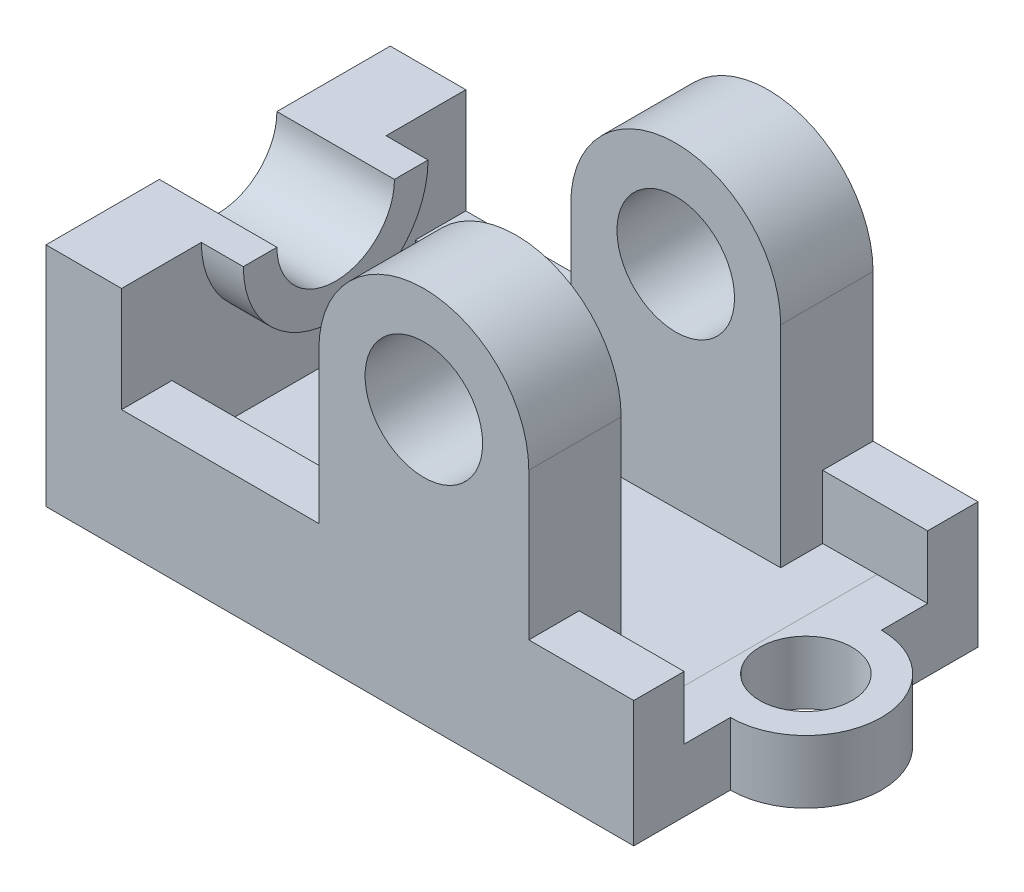
ISO-10303-21;
HEADER;
FILE_DESCRIPTION(('STEP AP214'),'2;1');
FILE_NAME('part.step','',(''),(''),'','','');
FILE_SCHEMA(('AUTOMOTIVE_DESIGN { 1 0 10303 214 1 1 1 1 }'));
ENDSEC;
DATA;
#1=APPLICATION_CONTEXT('core data for automotive mechanical design processes');
#2=APPLICATION_PROTOCOL_DEFINITION('international standard','automotive_design',2000,#1);
#3=PRODUCT_CONTEXT('',#1,'mechanical');
#4=PRODUCT('Part','Part','',(#3));
#5=PRODUCT_RELATED_PRODUCT_CATEGORY('part','',(#4));
#6=PRODUCT_DEFINITION_FORMATION('','',#4);
#7=PRODUCT_DEFINITION_CONTEXT('part definition',#1,'design');
#8=PRODUCT_DEFINITION('design','',#6,#7);
#9=PRODUCT_DEFINITION_SHAPE('','',#8);
#10=(LENGTH_UNIT() NAMED_UNIT(*) SI_UNIT(.MILLI.,.METRE.));
#11=(NAMED_UNIT(*) PLANE_ANGLE_UNIT() SI_UNIT($,.RADIAN.));
#12=(NAMED_UNIT(*) SI_UNIT($,.STERADIAN.) SOLID_ANGLE_UNIT());
#13=UNCERTAINTY_MEASURE_WITH_UNIT(LENGTH_MEASURE(1.E-05),#10,'distance_accuracy_value','');
#14=(GEOMETRIC_REPRESENTATION_CONTEXT(3) GLOBAL_UNCERTAINTY_ASSIGNED_CONTEXT((#13)) GLOBAL_UNIT_ASSIGNED_CONTEXT((#10,
#11,#12)) REPRESENTATION_CONTEXT('',''));
#15=CARTESIAN_POINT('',(0.,0.,0.));
#16=DIRECTION('',(0.,0.,1.));
#17=DIRECTION('',(1.,0.,0.));
#18=AXIS2_PLACEMENT_3D('',#15,#16,#17);
#19=CARTESIAN_POINT('',(0.,54.,82.));
#20=DIRECTION('',(0.,1.,0.));
#21=DIRECTION('',(0.,0.,1.));
#22=AXIS2_PLACEMENT_3D('',#19,#20,#21);
#23=PLANE('',#22);
#24=DIRECTION('',(-1.,0.,0.));
#25=VECTOR('',#24,1.);
#26=CARTESIAN_POINT('',(28.,54.,27.));
#27=LINE('',#26,#25);
#28=CARTESIAN_POINT('',(28.,54.,27.));
#29=VERTEX_POINT('',#28);
#30=CARTESIAN_POINT('',(0.,54.,27.));
#31=VERTEX_POINT('',#30);
#32=EDGE_CURVE('E237',#29,#31,#27,.T.);
#33=ORIENTED_EDGE('',*,*,#32,.F.);
#34=DIRECTION('',(0.,0.,1.));
#35=VECTOR('',#34,1.);
#36=CARTESIAN_POINT('',(28.,54.,63.));
#37=LINE('',#36,#35);
#38=CARTESIAN_POINT('',(28.,54.,19.));
#39=VERTEX_POINT('',#38);
#40=EDGE_CURVE('E247',#39,#29,#37,.T.);
#41=ORIENTED_EDGE('',*,*,#40,.F.);
#42=DIRECTION('',(-1.,0.,0.));
#43=VECTOR('',#42,1.);
#44=CARTESIAN_POINT('',(28.,54.,19.));
#45=LINE('',#44,#43);
#46=CARTESIAN_POINT('',(18.,54.,19.));
#47=VERTEX_POINT('',#46);
#48=EDGE_CURVE('E258',#39,#47,#45,.T.);
#49=ORIENTED_EDGE('',*,*,#48,.T.);
#50=DIRECTION('',(0.,0.,-1.));
#51=VECTOR('',#50,1.);
#52=CARTESIAN_POINT('',(18.,54.,82.));
#53=LINE('',#52,#51);
#54=CARTESIAN_POINT('',(18.,54.,0.));
#55=VERTEX_POINT('',#54);
#56=EDGE_CURVE('E478',#47,#55,#53,.T.);
#57=ORIENTED_EDGE('',*,*,#56,.T.);
#58=DIRECTION('',(1.,0.,0.));
#59=VECTOR('',#58,1.);
#60=CARTESIAN_POINT('',(0.,54.,0.));
#61=LINE('',#60,#59);
#62=CARTESIAN_POINT('',(0.,54.,0.));
#63=VERTEX_POINT('',#62);
#64=EDGE_CURVE('E464',#63,#55,#61,.T.);
#65=ORIENTED_EDGE('',*,*,#64,.F.);
#66=DIRECTION('',(0.,0.,-1.));
#67=VECTOR('',#66,1.);
#68=CARTESIAN_POINT('',(0.,54.,82.));
#69=LINE('',#68,#67);
#70=EDGE_CURVE('E252',#31,#63,#69,.T.);
#71=ORIENTED_EDGE('',*,*,#70,.F.);
#72=EDGE_LOOP('',(#33,#41,#49,#57,#65,#71));
#73=FACE_BOUND('',#72,.T.);
#74=ADVANCED_FACE('F50',(#73),#23,.T.);
#75=CARTESIAN_POINT('',(18.,0.,82.));
#76=DIRECTION('',(1.,0.,0.));
#77=DIRECTION('',(0.,1.,0.));
#78=AXIS2_PLACEMENT_3D('',#75,#76,#77);
#79=PLANE('',#78);
#80=ORIENTED_EDGE('',*,*,#56,.F.);
#81=CARTESIAN_POINT('',(18.,54.,41.));
#82=DIRECTION('',(1.,0.,0.));
#83=DIRECTION('',(0.,1.,0.));
#84=AXIS2_PLACEMENT_3D('',#81,#82,#83);
#85=CIRCLE('',#84,22.);
#86=CARTESIAN_POINT('',(18.,54.,63.));
#87=VERTEX_POINT('',#86);
#88=EDGE_CURVE('E71',#87,#47,#85,.T.);
#89=ORIENTED_EDGE('',*,*,#88,.F.);
#90=CARTESIAN_POINT('',(18.,54.,82.));
#91=VERTEX_POINT('',#90);
#92=EDGE_CURVE('E57',#91,#87,#53,.T.);
#93=ORIENTED_EDGE('',*,*,#92,.F.);
#94=DIRECTION('',(0.,-1.,0.));
#95=VECTOR('',#94,1.);
#96=CARTESIAN_POINT('',(18.,0.,82.));
#97=LINE('',#96,#95);
#98=CARTESIAN_POINT('',(18.,29.,82.));
#99=VERTEX_POINT('',#98);
#100=EDGE_CURVE('E446',#91,#99,#97,.T.);
#101=ORIENTED_EDGE('',*,*,#100,.T.);
#102=DIRECTION('',(0.,0.,1.));
#103=VECTOR('',#102,1.);
#104=CARTESIAN_POINT('',(18.,29.,70.));
#105=LINE('',#104,#103);
#106=CARTESIAN_POINT('',(18.,29.,70.));
#107=VERTEX_POINT('',#106);
#108=EDGE_CURVE('E308',#107,#99,#105,.T.);
#109=ORIENTED_EDGE('',*,*,#108,.F.);
#110=DIRECTION('',(0.,-1.,0.));
#111=VECTOR('',#110,1.);
#112=CARTESIAN_POINT('',(18.,14.,70.));
#113=LINE('',#112,#111);
#114=CARTESIAN_POINT('',(18.,14.,70.));
#115=VERTEX_POINT('',#114);
#116=EDGE_CURVE('E305',#107,#115,#113,.T.);
#117=ORIENTED_EDGE('',*,*,#116,.T.);
#118=DIRECTION('',(0.,0.,-1.));
#119=VECTOR('',#118,1.);
#120=CARTESIAN_POINT('',(18.,14.,82.));
#121=LINE('',#120,#119);
#122=CARTESIAN_POINT('',(18.,14.,12.));
#123=VERTEX_POINT('',#122);
#124=EDGE_CURVE('E11',#115,#123,#121,.T.);
#125=ORIENTED_EDGE('',*,*,#124,.T.);
#126=DIRECTION('',(0.,1.,0.));
#127=VECTOR('',#126,1.);
#128=CARTESIAN_POINT('',(18.,14.,12.));
#129=LINE('',#128,#127);
#130=CARTESIAN_POINT('',(18.,29.,12.));
#131=VERTEX_POINT('',#130);
#132=EDGE_CURVE('E363',#123,#131,#129,.T.);
#133=ORIENTED_EDGE('',*,*,#132,.T.);
#134=DIRECTION('',(0.,0.,-1.));
#135=VECTOR('',#134,1.);
#136=CARTESIAN_POINT('',(18.,29.,12.));
#137=LINE('',#136,#135);
#138=CARTESIAN_POINT('',(18.,29.,0.));
#139=VERTEX_POINT('',#138);
#140=EDGE_CURVE('E367',#131,#139,#137,.T.);
#141=ORIENTED_EDGE('',*,*,#140,.T.);
#142=DIRECTION('',(0.,-1.,0.));
#143=VECTOR('',#142,1.);
#144=CARTESIAN_POINT('',(18.,0.,0.));
#145=LINE('',#144,#143);
#146=EDGE_CURVE('E443',#55,#139,#145,.T.);
#147=ORIENTED_EDGE('',*,*,#146,.F.);
#148=EDGE_LOOP('',(#80,#89,#93,#101,#109,#117,#125,#133,#141,#147));
#149=FACE_BOUND('',#148,.T.);
#150=ADVANCED_FACE('F484',(#149),#79,.T.);
#151=CARTESIAN_POINT('',(140.,0.,0.));
#152=DIRECTION('',(1.,0.,0.));
#153=DIRECTION('',(0.,0.,-1.));
#154=AXIS2_PLACEMENT_3D('',#151,#152,#153);
#155=PLANE('',#154);
#156=DIRECTION('',(0.,1.,0.));
#157=VECTOR('',#156,1.);
#158=CARTESIAN_POINT('',(140.,0.,23.));
#159=LINE('',#158,#157);
#160=CARTESIAN_POINT('',(140.,0.,23.));
#161=VERTEX_POINT('',#160);
#162=CARTESIAN_POINT('',(140.,15.,23.));
#163=VERTEX_POINT('',#162);
#164=EDGE_CURVE('E276',#161,#163,#159,.T.);
#165=ORIENTED_EDGE('',*,*,#164,.F.);
#166=DIRECTION('',(0.,0.,1.));
#167=VECTOR('',#166,1.);
#168=CARTESIAN_POINT('',(140.,0.,0.));
#169=LINE('',#168,#167);
#170=CARTESIAN_POINT('',(140.,0.,0.));
#171=VERTEX_POINT('',#170);
#172=EDGE_CURVE('E447',#171,#161,#169,.T.);
#173=ORIENTED_EDGE('',*,*,#172,.F.);
#174=DIRECTION('',(0.,1.,0.));
#175=VECTOR('',#174,1.);
#176=CARTESIAN_POINT('',(140.,0.,0.));
#177=LINE('',#176,#175);
#178=CARTESIAN_POINT('',(140.,30.,0.));
#179=VERTEX_POINT('',#178);
#180=EDGE_CURVE('E438',#171,#179,#177,.T.);
#181=ORIENTED_EDGE('',*,*,#180,.T.);
#182=DIRECTION('',(0.,0.,-1.));
#183=VECTOR('',#182,1.);
#184=CARTESIAN_POINT('',(140.,30.,12.));
#185=LINE('',#184,#183);
#186=CARTESIAN_POINT('',(140.,30.,12.));
#187=VERTEX_POINT('',#186);
#188=EDGE_CURVE('E350',#187,#179,#185,.T.);
#189=ORIENTED_EDGE('',*,*,#188,.F.);
#190=DIRECTION('',(0.,-1.,0.));
#191=VECTOR('',#190,1.);
#192=CARTESIAN_POINT('',(140.,15.,12.));
#193=LINE('',#192,#191);
#194=CARTESIAN_POINT('',(140.,15.,12.));
#195=VERTEX_POINT('',#194);
#196=EDGE_CURVE('E341',#187,#195,#193,.T.);
#197=ORIENTED_EDGE('',*,*,#196,.T.);
#198=DIRECTION('',(0.,0.,1.));
#199=VECTOR('',#198,1.);
#200=CARTESIAN_POINT('',(140.,15.,0.));
#201=LINE('',#200,#199);
#202=EDGE_CURVE('E445',#195,#163,#201,.T.);
#203=ORIENTED_EDGE('',*,*,#202,.T.);
#204=EDGE_LOOP('',(#165,#173,#181,#189,#197,#203));
#205=FACE_BOUND('',#204,.T.);
#206=ADVANCED_FACE('F513',(#205),#155,.T.);
#207=CARTESIAN_POINT('',(-0.12577472936121,13.8352202297331,82.));
#208=DIRECTION('',(-0.00909053345679159,0.999958680247074,0.));
#209=DIRECTION('',(-0.999958680247075,-0.00909053345679159,0.));
#210=AXIS2_PLACEMENT_3D('',#207,#208,#209);
#211=PLANE('',#210);
#212=DIRECTION('',(0.999958680247074,0.0090905334567916,0.));
#213=VECTOR('',#212,1.);
#214=CARTESIAN_POINT('',(65.,14.4272727272727,70.));
#215=LINE('',#214,#213);
#216=CARTESIAN_POINT('',(65.,14.4272727272727,70.));
#217=VERTEX_POINT('',#216);
#218=EDGE_CURVE('E295',#115,#217,#215,.T.);
#219=ORIENTED_EDGE('',*,*,#218,.T.);
#220=DIRECTION('',(0.,0.,1.));
#221=VECTOR('',#220,1.);
#222=CARTESIAN_POINT('',(65.,14.4272727272727,60.));
#223=LINE('',#222,#221);
#224=CARTESIAN_POINT('',(65.,14.4272727272727,60.));
#225=VERTEX_POINT('',#224);
#226=EDGE_CURVE('E435',#225,#217,#223,.T.);
#227=ORIENTED_EDGE('',*,*,#226,.F.);
#228=DIRECTION('',(-0.999958680247075,-0.0090905334567916,0.));
#229=VECTOR('',#228,1.);
#230=CARTESIAN_POINT('',(-0.12577472936121,13.8352202297331,60.));
#231=LINE('',#230,#229);
#232=CARTESIAN_POINT('',(115.,14.8818181818182,60.));
#233=VERTEX_POINT('',#232);
#234=EDGE_CURVE('E417',#233,#225,#231,.T.);
#235=ORIENTED_EDGE('',*,*,#234,.F.);
#236=DIRECTION('',(0.,0.,1.));
#237=VECTOR('',#236,1.);
#238=CARTESIAN_POINT('',(115.,14.8818181818182,60.));
#239=LINE('',#238,#237);
#240=CARTESIAN_POINT('',(115.,14.8818181818182,70.));
#241=VERTEX_POINT('',#240);
#242=EDGE_CURVE('E426',#233,#241,#239,.T.);
#243=ORIENTED_EDGE('',*,*,#242,.T.);
#244=DIRECTION('',(0.999958680247075,0.00909053345679159,0.));
#245=VECTOR('',#244,1.);
#246=CARTESIAN_POINT('',(-0.12577472936121,13.8352202297331,70.));
#247=LINE('',#246,#245);
#248=CARTESIAN_POINT('',(128.,15.,70.));
#249=VERTEX_POINT('',#248);
#250=EDGE_CURVE('E335',#241,#249,#247,.T.);
#251=ORIENTED_EDGE('',*,*,#250,.T.);
#252=DIRECTION('',(0.,0.,-1.));
#253=VECTOR('',#252,1.);
#254=CARTESIAN_POINT('',(128.,15.,82.));
#255=LINE('',#254,#253);
#256=CARTESIAN_POINT('',(128.,15.,12.));
#257=VERTEX_POINT('',#256);
#258=EDGE_CURVE('E465',#249,#257,#255,.T.);
#259=ORIENTED_EDGE('',*,*,#258,.T.);
#260=DIRECTION('',(0.999958680247075,0.00909053345679159,0.));
#261=VECTOR('',#260,1.);
#262=CARTESIAN_POINT('',(-0.12577472936121,13.8352202297331,12.));
#263=LINE('',#262,#261);
#264=CARTESIAN_POINT('',(115.,14.8818181818182,12.));
#265=VERTEX_POINT('',#264);
#266=EDGE_CURVE('E353',#265,#257,#263,.T.);
#267=ORIENTED_EDGE('',*,*,#266,.F.);
#268=DIRECTION('',(0.,0.,-1.));
#269=VECTOR('',#268,1.);
#270=CARTESIAN_POINT('',(115.,14.8818181818182,22.));
#271=LINE('',#270,#269);
#272=CARTESIAN_POINT('',(115.,14.8818181818182,22.));
#273=VERTEX_POINT('',#272);
#274=EDGE_CURVE('E404',#273,#265,#271,.T.);
#275=ORIENTED_EDGE('',*,*,#274,.F.);
#276=DIRECTION('',(-0.999958680247075,-0.00909053345679171,0.));
#277=VECTOR('',#276,1.);
#278=CARTESIAN_POINT('',(115.,14.8818181818182,22.));
#279=LINE('',#278,#277);
#280=CARTESIAN_POINT('',(65.,14.4272727272727,22.));
#281=VERTEX_POINT('',#280);
#282=EDGE_CURVE('E381',#273,#281,#279,.T.);
#283=ORIENTED_EDGE('',*,*,#282,.T.);
#284=DIRECTION('',(0.,0.,-1.));
#285=VECTOR('',#284,1.);
#286=CARTESIAN_POINT('',(65.,14.4272727272727,22.));
#287=LINE('',#286,#285);
#288=CARTESIAN_POINT('',(65.,14.4272727272727,12.));
#289=VERTEX_POINT('',#288);
#290=EDGE_CURVE('E402',#281,#289,#287,.T.);
#291=ORIENTED_EDGE('',*,*,#290,.T.);
#292=DIRECTION('',(-0.999958680247075,-0.0090905334567916,0.));
#293=VECTOR('',#292,1.);
#294=CARTESIAN_POINT('',(65.,14.4272727272727,12.));
#295=LINE('',#294,#293);
#296=EDGE_CURVE('E356',#289,#123,#295,.T.);
#297=ORIENTED_EDGE('',*,*,#296,.T.);
#298=ORIENTED_EDGE('',*,*,#124,.F.);
#299=EDGE_LOOP('',(#219,#227,#235,#243,#251,#259,#267,#275,#283,#291,#297,#298));
#300=FACE_BOUND('',#299,.T.);
#301=ADVANCED_FACE('F47',(#300),#211,.T.);
#302=CARTESIAN_POINT('',(140.,15.,0.));
#303=DIRECTION('',(0.,1.,0.));
#304=DIRECTION('',(0.,0.,1.));
#305=AXIS2_PLACEMENT_3D('',#302,#303,#304);
#306=PLANE('',#305);
#307=CARTESIAN_POINT('',(140.,15.,41.));
#308=DIRECTION('',(0.,1.,0.));
#309=DIRECTION('',(0.,0.,1.));
#310=AXIS2_PLACEMENT_3D('',#307,#308,#309);
#311=CIRCLE('',#310,11.);
#312=CARTESIAN_POINT('',(140.,15.,52.));
#313=VERTEX_POINT('',#312);
#314=EDGE_CURVE('E266',#313,#313,#311,.T.);
#315=ORIENTED_EDGE('',*,*,#314,.F.);
#316=EDGE_LOOP('',(#315));
#317=FACE_BOUND('',#316,.T.);
#318=ORIENTED_EDGE('',*,*,#258,.F.);
#319=DIRECTION('',(1.,0.,0.));
#320=VECTOR('',#319,1.);
#321=CARTESIAN_POINT('',(140.,15.,70.));
#322=LINE('',#321,#320);
#323=CARTESIAN_POINT('',(140.,15.,70.));
#324=VERTEX_POINT('',#323);
#325=EDGE_CURVE('E330',#249,#324,#322,.T.);
#326=ORIENTED_EDGE('',*,*,#325,.T.);
#327=CARTESIAN_POINT('',(140.,15.,59.));
#328=VERTEX_POINT('',#327);
#329=EDGE_CURVE('E444',#328,#324,#201,.T.);
#330=ORIENTED_EDGE('',*,*,#329,.F.);
#331=CARTESIAN_POINT('',(140.,15.,41.));
#332=DIRECTION('',(0.,1.,0.));
#333=DIRECTION('',(0.,0.,1.));
#334=AXIS2_PLACEMENT_3D('',#331,#332,#333);
#335=CIRCLE('',#334,18.);
#336=EDGE_CURVE('E269',#328,#163,#335,.T.);
#337=ORIENTED_EDGE('',*,*,#336,.T.);
#338=ORIENTED_EDGE('',*,*,#202,.F.);
#339=DIRECTION('',(1.,0.,0.));
#340=VECTOR('',#339,1.);
#341=CARTESIAN_POINT('',(140.,15.,12.));
#342=LINE('',#341,#340);
#343=EDGE_CURVE('E346',#257,#195,#342,.T.);
#344=ORIENTED_EDGE('',*,*,#343,.F.);
#345=EDGE_LOOP('',(#318,#326,#330,#337,#338,#344));
#346=FACE_BOUND('',#345,.T.);
#347=ADVANCED_FACE('F520',(#317,#346),#306,.T.);
#348=DIRECTION('',(-1.,0.,0.));
#349=VECTOR('',#348,1.);
#350=CARTESIAN_POINT('',(28.,54.,55.));
#351=LINE('',#350,#349);
#352=CARTESIAN_POINT('',(28.,54.,55.));
#353=VERTEX_POINT('',#352);
#354=CARTESIAN_POINT('',(0.,54.,55.));
#355=VERTEX_POINT('',#354);
#356=EDGE_CURVE('E62',#353,#355,#351,.T.);
#357=ORIENTED_EDGE('',*,*,#356,.T.);
#358=CARTESIAN_POINT('',(0.,54.,82.));
#359=VERTEX_POINT('',#358);
#360=EDGE_CURVE('E474',#359,#355,#69,.T.);
#361=ORIENTED_EDGE('',*,*,#360,.F.);
#362=DIRECTION('',(1.,0.,0.));
#363=VECTOR('',#362,1.);
#364=CARTESIAN_POINT('',(0.,54.,82.));
#365=LINE('',#364,#363);
#366=EDGE_CURVE('E455',#359,#91,#365,.T.);
#367=ORIENTED_EDGE('',*,*,#366,.T.);
#368=ORIENTED_EDGE('',*,*,#92,.T.);
#369=DIRECTION('',(-1.,0.,0.));
#370=VECTOR('',#369,1.);
#371=CARTESIAN_POINT('',(28.,54.,63.));
#372=LINE('',#371,#370);
#373=CARTESIAN_POINT('',(28.,54.,63.));
#374=VERTEX_POINT('',#373);
#375=EDGE_CURVE('E256',#374,#87,#372,.T.);
#376=ORIENTED_EDGE('',*,*,#375,.F.);
#377=EDGE_CURVE('E260',#353,#374,#37,.T.);
#378=ORIENTED_EDGE('',*,*,#377,.F.);
#379=EDGE_LOOP('',(#357,#361,#367,#368,#376,#378));
#380=FACE_BOUND('',#379,.T.);
#381=ADVANCED_FACE('F492',(#380),#23,.T.);
#382=CARTESIAN_POINT('',(0.,0.,82.));
#383=DIRECTION('',(-1.,0.,0.));
#384=DIRECTION('',(0.,0.,1.));
#385=AXIS2_PLACEMENT_3D('',#382,#383,#384);
#386=PLANE('',#385);
#387=CARTESIAN_POINT('',(0.,54.,41.));
#388=DIRECTION('',(-1.,0.,0.));
#389=DIRECTION('',(0.,0.,1.));
#390=AXIS2_PLACEMENT_3D('',#387,#388,#389);
#391=CIRCLE('',#390,14.);
#392=EDGE_CURVE('E242',#31,#355,#391,.T.);
#393=ORIENTED_EDGE('',*,*,#392,.F.);
#394=ORIENTED_EDGE('',*,*,#70,.T.);
#395=DIRECTION('',(0.,1.,0.));
#396=VECTOR('',#395,1.);
#397=CARTESIAN_POINT('',(0.,0.,0.));
#398=LINE('',#397,#396);
#399=CARTESIAN_POINT('',(0.,0.,0.));
#400=VERTEX_POINT('',#399);
#401=EDGE_CURVE('E466',#400,#63,#398,.T.);
#402=ORIENTED_EDGE('',*,*,#401,.F.);
#403=DIRECTION('',(0.,0.,-1.));
#404=VECTOR('',#403,1.);
#405=CARTESIAN_POINT('',(0.,0.,82.));
#406=LINE('',#405,#404);
#407=CARTESIAN_POINT('',(0.,0.,82.));
#408=VERTEX_POINT('',#407);
#409=EDGE_CURVE('E472',#408,#400,#406,.T.);
#410=ORIENTED_EDGE('',*,*,#409,.F.);
#411=DIRECTION('',(0.,1.,0.));
#412=VECTOR('',#411,1.);
#413=CARTESIAN_POINT('',(0.,0.,82.));
#414=LINE('',#413,#412);
#415=EDGE_CURVE('E457',#408,#359,#414,.T.);
#416=ORIENTED_EDGE('',*,*,#415,.T.);
#417=ORIENTED_EDGE('',*,*,#360,.T.);
#418=EDGE_LOOP('',(#393,#394,#402,#410,#416,#417));
#419=FACE_BOUND('',#418,.T.);
#420=ADVANCED_FACE('F495',(#419),#386,.T.);
#421=CARTESIAN_POINT('',(0.,0.,82.));
#422=DIRECTION('',(0.,1.,0.));
#423=DIRECTION('',(0.,0.,1.));
#424=AXIS2_PLACEMENT_3D('',#421,#422,#423);
#425=PLANE('',#424);
#426=CARTESIAN_POINT('',(140.,0.,41.));
#427=DIRECTION('',(0.,1.,0.));
#428=DIRECTION('',(0.,0.,1.));
#429=AXIS2_PLACEMENT_3D('',#426,#427,#428);
#430=CIRCLE('',#429,11.);
#431=CARTESIAN_POINT('',(140.,0.,52.));
#432=VERTEX_POINT('',#431);
#433=EDGE_CURVE('E270',#432,#432,#430,.T.);
#434=ORIENTED_EDGE('',*,*,#433,.T.);
#435=EDGE_LOOP('',(#434));
#436=FACE_BOUND('',#435,.T.);
#437=DIRECTION('',(1.,0.,0.));
#438=VECTOR('',#437,1.);
#439=CARTESIAN_POINT('',(0.,0.,0.));
#440=LINE('',#439,#438);
#441=EDGE_CURVE('E452',#400,#171,#440,.T.);
#442=ORIENTED_EDGE('',*,*,#441,.T.);
#443=ORIENTED_EDGE('',*,*,#172,.T.);
#444=CARTESIAN_POINT('',(140.,0.,41.));
#445=DIRECTION('',(0.,1.,0.));
#446=DIRECTION('',(0.,0.,1.));
#447=AXIS2_PLACEMENT_3D('',#444,#445,#446);
#448=CIRCLE('',#447,18.);
#449=CARTESIAN_POINT('',(140.,0.,59.));
#450=VERTEX_POINT('',#449);
#451=EDGE_CURVE('E271',#450,#161,#448,.T.);
#452=ORIENTED_EDGE('',*,*,#451,.F.);
#453=CARTESIAN_POINT('',(140.,0.,82.));
#454=VERTEX_POINT('',#453);
#455=EDGE_CURVE('E439',#450,#454,#169,.T.);
#456=ORIENTED_EDGE('',*,*,#455,.T.);
#457=DIRECTION('',(1.,0.,0.));
#458=VECTOR('',#457,1.);
#459=CARTESIAN_POINT('',(0.,0.,82.));
#460=LINE('',#459,#458);
#461=EDGE_CURVE('E459',#408,#454,#460,.T.);
#462=ORIENTED_EDGE('',*,*,#461,.F.);
#463=ORIENTED_EDGE('',*,*,#409,.T.);
#464=EDGE_LOOP('',(#442,#443,#452,#456,#462,#463));
#465=FACE_BOUND('',#464,.T.);
#466=ADVANCED_FACE('F525',(#436,#465),#425,.F.);
#467=CARTESIAN_POINT('',(0.,0.,82.));
#468=DIRECTION('',(0.,0.,1.));
#469=DIRECTION('',(1.,0.,0.));
#470=AXIS2_PLACEMENT_3D('',#467,#468,#469);
#471=PLANE('',#470);
#472=CARTESIAN_POINT('',(90.,65.,82.));
#473=DIRECTION('',(0.,0.,1.));
#474=DIRECTION('',(1.,0.,0.));
#475=AXIS2_PLACEMENT_3D('',#472,#473,#474);
#476=CIRCLE('',#475,14.);
#477=CARTESIAN_POINT('',(104.,65.,82.));
#478=VERTEX_POINT('',#477);
#479=EDGE_CURVE('E285',#478,#478,#476,.T.);
#480=ORIENTED_EDGE('',*,*,#479,.F.);
#481=EDGE_LOOP('',(#480));
#482=FACE_BOUND('',#481,.T.);
#483=DIRECTION('',(0.,1.,0.));
#484=VECTOR('',#483,1.);
#485=CARTESIAN_POINT('',(140.,0.,82.));
#486=LINE('',#485,#484);
#487=CARTESIAN_POINT('',(140.,30.,82.));
#488=VERTEX_POINT('',#487);
#489=EDGE_CURVE('E431',#454,#488,#486,.T.);
#490=ORIENTED_EDGE('',*,*,#489,.T.);
#491=DIRECTION('',(-1.,0.,0.));
#492=VECTOR('',#491,1.);
#493=CARTESIAN_POINT('',(140.,30.,82.));
#494=LINE('',#493,#492);
#495=CARTESIAN_POINT('',(115.,30.,82.));
#496=VERTEX_POINT('',#495);
#497=EDGE_CURVE('E309',#488,#496,#494,.T.);
#498=ORIENTED_EDGE('',*,*,#497,.T.);
#499=DIRECTION('',(0.,-1.,0.));
#500=VECTOR('',#499,1.);
#501=CARTESIAN_POINT('',(115.,0.,82.));
#502=LINE('',#501,#500);
#503=CARTESIAN_POINT('',(115.,65.,82.));
#504=VERTEX_POINT('',#503);
#505=EDGE_CURVE('E399',#504,#496,#502,.T.);
#506=ORIENTED_EDGE('',*,*,#505,.F.);
#507=CARTESIAN_POINT('',(90.,65.,82.));
#508=DIRECTION('',(0.,0.,1.));
#509=DIRECTION('',(1.,0.,0.));
#510=AXIS2_PLACEMENT_3D('',#507,#508,#509);
#511=CIRCLE('',#510,25.);
#512=CARTESIAN_POINT('',(65.,65.,82.));
#513=VERTEX_POINT('',#512);
#514=EDGE_CURVE('E421',#504,#513,#511,.T.);
#515=ORIENTED_EDGE('',*,*,#514,.T.);
#516=DIRECTION('',(0.,-1.,0.));
#517=VECTOR('',#516,1.);
#518=CARTESIAN_POINT('',(65.,0.,82.));
#519=LINE('',#518,#517);
#520=CARTESIAN_POINT('',(65.,29.,82.));
#521=VERTEX_POINT('',#520);
#522=EDGE_CURVE('E415',#513,#521,#519,.T.);
#523=ORIENTED_EDGE('',*,*,#522,.T.);
#524=DIRECTION('',(-1.,0.,0.));
#525=VECTOR('',#524,1.);
#526=CARTESIAN_POINT('',(18.,29.,82.));
#527=LINE('',#526,#525);
#528=EDGE_CURVE('E291',#521,#99,#527,.T.);
#529=ORIENTED_EDGE('',*,*,#528,.T.);
#530=ORIENTED_EDGE('',*,*,#100,.F.);
#531=ORIENTED_EDGE('',*,*,#366,.F.);
#532=ORIENTED_EDGE('',*,*,#415,.F.);
#533=ORIENTED_EDGE('',*,*,#461,.T.);
#534=EDGE_LOOP('',(#490,#498,#506,#515,#523,#529,#530,#531,#532,#533));
#535=FACE_BOUND('',#534,.T.);
#536=ADVANCED_FACE('F545',(#482,#535),#471,.T.);
#537=CARTESIAN_POINT('',(0.,0.,0.));
#538=DIRECTION('',(0.,0.,1.));
#539=DIRECTION('',(1.,0.,0.));
#540=AXIS2_PLACEMENT_3D('',#537,#538,#539);
#541=PLANE('',#540);
#542=CARTESIAN_POINT('',(90.,65.,0.));
#543=DIRECTION('',(0.,0.,1.));
#544=DIRECTION('',(1.,0.,0.));
#545=AXIS2_PLACEMENT_3D('',#542,#543,#544);
#546=CIRCLE('',#545,14.);
#547=CARTESIAN_POINT('',(104.,65.,0.));
#548=VERTEX_POINT('',#547);
#549=EDGE_CURVE('E289',#548,#548,#546,.T.);
#550=ORIENTED_EDGE('',*,*,#549,.T.);
#551=EDGE_LOOP('',(#550));
#552=FACE_BOUND('',#551,.T.);
#553=DIRECTION('',(1.,0.,0.));
#554=VECTOR('',#553,1.);
#555=CARTESIAN_POINT('',(140.,30.,0.));
#556=LINE('',#555,#554);
#557=CARTESIAN_POINT('',(115.,30.,0.));
#558=VERTEX_POINT('',#557);
#559=EDGE_CURVE('E333',#558,#179,#556,.T.);
#560=ORIENTED_EDGE('',*,*,#559,.T.);
#561=ORIENTED_EDGE('',*,*,#180,.F.);
#562=ORIENTED_EDGE('',*,*,#441,.F.);
#563=ORIENTED_EDGE('',*,*,#401,.T.);
#564=ORIENTED_EDGE('',*,*,#64,.T.);
#565=ORIENTED_EDGE('',*,*,#146,.T.);
#566=DIRECTION('',(1.,0.,0.));
#567=VECTOR('',#566,1.);
#568=CARTESIAN_POINT('',(18.,29.,0.));
#569=LINE('',#568,#567);
#570=CARTESIAN_POINT('',(65.,29.,0.));
#571=VERTEX_POINT('',#570);
#572=EDGE_CURVE('E357',#139,#571,#569,.T.);
#573=ORIENTED_EDGE('',*,*,#572,.T.);
#574=DIRECTION('',(0.,1.,0.));
#575=VECTOR('',#574,1.);
#576=CARTESIAN_POINT('',(65.,14.4272727272727,0.));
#577=LINE('',#576,#575);
#578=CARTESIAN_POINT('',(65.,65.,0.));
#579=VERTEX_POINT('',#578);
#580=EDGE_CURVE('E382',#571,#579,#577,.T.);
#581=ORIENTED_EDGE('',*,*,#580,.T.);
#582=CARTESIAN_POINT('',(90.,65.,0.));
#583=DIRECTION('',(0.,0.,-1.));
#584=DIRECTION('',(-1.,0.,0.));
#585=AXIS2_PLACEMENT_3D('',#582,#583,#584);
#586=CIRCLE('',#585,25.);
#587=CARTESIAN_POINT('',(115.,65.,0.));
#588=VERTEX_POINT('',#587);
#589=EDGE_CURVE('E372',#579,#588,#586,.T.);
#590=ORIENTED_EDGE('',*,*,#589,.T.);
#591=DIRECTION('',(0.,-1.,0.));
#592=VECTOR('',#591,1.);
#593=CARTESIAN_POINT('',(115.,65.,0.));
#594=LINE('',#593,#592);
#595=EDGE_CURVE('E393',#588,#558,#594,.T.);
#596=ORIENTED_EDGE('',*,*,#595,.T.);
#597=EDGE_LOOP('',(#560,#561,#562,#563,#564,#565,#573,#581,#590,#596));
#598=FACE_BOUND('',#597,.T.);
#599=ADVANCED_FACE('F487',(#552,#598),#541,.F.);
#600=DIRECTION('',(0.,1.,0.));
#601=VECTOR('',#600,1.);
#602=CARTESIAN_POINT('',(140.,0.,59.));
#603=LINE('',#602,#601);
#604=EDGE_CURVE('E278',#450,#328,#603,.T.);
#605=ORIENTED_EDGE('',*,*,#604,.T.);
#606=ORIENTED_EDGE('',*,*,#329,.T.);
#607=DIRECTION('',(0.,1.,0.));
#608=VECTOR('',#607,1.);
#609=CARTESIAN_POINT('',(140.,15.,70.));
#610=LINE('',#609,#608);
#611=CARTESIAN_POINT('',(140.,30.,70.));
#612=VERTEX_POINT('',#611);
#613=EDGE_CURVE('E319',#324,#612,#610,.T.);
#614=ORIENTED_EDGE('',*,*,#613,.T.);
#615=DIRECTION('',(0.,0.,1.));
#616=VECTOR('',#615,1.);
#617=CARTESIAN_POINT('',(140.,30.,70.));
#618=LINE('',#617,#616);
#619=EDGE_CURVE('E323',#612,#488,#618,.T.);
#620=ORIENTED_EDGE('',*,*,#619,.T.);
#621=ORIENTED_EDGE('',*,*,#489,.F.);
#622=ORIENTED_EDGE('',*,*,#455,.F.);
#623=EDGE_LOOP('',(#605,#606,#614,#620,#621,#622));
#624=FACE_BOUND('',#623,.T.);
#625=ADVANCED_FACE('F537',(#624),#155,.T.);
#626=CARTESIAN_POINT('',(115.,0.,60.));
#627=DIRECTION('',(-1.,0.,0.));
#628=DIRECTION('',(0.,0.,1.));
#629=AXIS2_PLACEMENT_3D('',#626,#627,#628);
#630=PLANE('',#629);
#631=ORIENTED_EDGE('',*,*,#505,.T.);
#632=DIRECTION('',(0.,0.,1.));
#633=VECTOR('',#632,1.);
#634=CARTESIAN_POINT('',(115.,30.,70.));
#635=LINE('',#634,#633);
#636=CARTESIAN_POINT('',(115.,30.,70.));
#637=VERTEX_POINT('',#636);
#638=EDGE_CURVE('E321',#637,#496,#635,.T.);
#639=ORIENTED_EDGE('',*,*,#638,.F.);
#640=DIRECTION('',(0.,-1.,0.));
#641=VECTOR('',#640,1.);
#642=CARTESIAN_POINT('',(115.,30.,70.));
#643=LINE('',#642,#641);
#644=EDGE_CURVE('E317',#637,#241,#643,.T.);
#645=ORIENTED_EDGE('',*,*,#644,.T.);
#646=ORIENTED_EDGE('',*,*,#242,.F.);
#647=DIRECTION('',(0.,-1.,0.));
#648=VECTOR('',#647,1.);
#649=CARTESIAN_POINT('',(115.,0.,60.));
#650=LINE('',#649,#648);
#651=CARTESIAN_POINT('',(115.,65.,60.));
#652=VERTEX_POINT('',#651);
#653=EDGE_CURVE('E407',#652,#233,#650,.T.);
#654=ORIENTED_EDGE('',*,*,#653,.F.);
#655=DIRECTION('',(0.,0.,1.));
#656=VECTOR('',#655,1.);
#657=CARTESIAN_POINT('',(115.,65.,60.));
#658=LINE('',#657,#656);
#659=EDGE_CURVE('E423',#652,#504,#658,.T.);
#660=ORIENTED_EDGE('',*,*,#659,.T.);
#661=EDGE_LOOP('',(#631,#639,#645,#646,#654,#660));
#662=FACE_BOUND('',#661,.T.);
#663=ADVANCED_FACE('F536',(#662),#630,.F.);
#664=CARTESIAN_POINT('',(65.,0.,60.));
#665=DIRECTION('',(-1.,0.,0.));
#666=DIRECTION('',(0.,0.,1.));
#667=AXIS2_PLACEMENT_3D('',#664,#665,#666);
#668=PLANE('',#667);
#669=DIRECTION('',(0.,0.,1.));
#670=VECTOR('',#669,1.);
#671=CARTESIAN_POINT('',(65.,29.,70.));
#672=LINE('',#671,#670);
#673=CARTESIAN_POINT('',(65.,29.,70.));
#674=VERTEX_POINT('',#673);
#675=EDGE_CURVE('E304',#674,#521,#672,.T.);
#676=ORIENTED_EDGE('',*,*,#675,.T.);
#677=ORIENTED_EDGE('',*,*,#522,.F.);
#678=DIRECTION('',(0.,0.,1.));
#679=VECTOR('',#678,1.);
#680=CARTESIAN_POINT('',(65.,65.,60.));
#681=LINE('',#680,#679);
#682=CARTESIAN_POINT('',(65.,65.,60.));
#683=VERTEX_POINT('',#682);
#684=EDGE_CURVE('E434',#683,#513,#681,.T.);
#685=ORIENTED_EDGE('',*,*,#684,.F.);
#686=DIRECTION('',(0.,-1.,0.));
#687=VECTOR('',#686,1.);
#688=CARTESIAN_POINT('',(65.,0.,60.));
#689=LINE('',#688,#687);
#690=EDGE_CURVE('E411',#683,#225,#689,.T.);
#691=ORIENTED_EDGE('',*,*,#690,.T.);
#692=ORIENTED_EDGE('',*,*,#226,.T.);
#693=DIRECTION('',(0.,1.,0.));
#694=VECTOR('',#693,1.);
#695=CARTESIAN_POINT('',(65.,29.,70.));
#696=LINE('',#695,#694);
#697=EDGE_CURVE('E300',#217,#674,#696,.T.);
#698=ORIENTED_EDGE('',*,*,#697,.T.);
#699=EDGE_LOOP('',(#676,#677,#685,#691,#692,#698));
#700=FACE_BOUND('',#699,.T.);
#701=ADVANCED_FACE('F597',(#700),#668,.T.);
#702=CARTESIAN_POINT('',(90.,65.,60.));
#703=DIRECTION('',(0.,0.,1.));
#704=DIRECTION('',(1.,0.,0.));
#705=AXIS2_PLACEMENT_3D('',#702,#703,#704);
#706=CYLINDRICAL_SURFACE('',#705,25.);
#707=ORIENTED_EDGE('',*,*,#514,.F.);
#708=ORIENTED_EDGE('',*,*,#659,.F.);
#709=CARTESIAN_POINT('',(90.,65.,60.));
#710=DIRECTION('',(0.,0.,1.));
#711=DIRECTION('',(1.,0.,0.));
#712=AXIS2_PLACEMENT_3D('',#709,#710,#711);
#713=CIRCLE('',#712,25.);
#714=EDGE_CURVE('E412',#652,#683,#713,.T.);
#715=ORIENTED_EDGE('',*,*,#714,.T.);
#716=ORIENTED_EDGE('',*,*,#684,.T.);
#717=EDGE_LOOP('',(#707,#708,#715,#716));
#718=FACE_BOUND('',#717,.T.);
#719=ADVANCED_FACE('F603',(#718),#706,.T.);
#720=CARTESIAN_POINT('',(0.,0.,60.));
#721=DIRECTION('',(0.,0.,1.));
#722=DIRECTION('',(1.,0.,0.));
#723=AXIS2_PLACEMENT_3D('',#720,#721,#722);
#724=PLANE('',#723);
#725=CARTESIAN_POINT('',(90.,65.,60.));
#726=DIRECTION('',(0.,0.,1.));
#727=DIRECTION('',(1.,0.,0.));
#728=AXIS2_PLACEMENT_3D('',#725,#726,#727);
#729=CIRCLE('',#728,14.);
#730=CARTESIAN_POINT('',(104.,65.,60.));
#731=VERTEX_POINT('',#730);
#732=EDGE_CURVE('E290',#731,#731,#729,.T.);
#733=ORIENTED_EDGE('',*,*,#732,.T.);
#734=EDGE_LOOP('',(#733));
#735=FACE_BOUND('',#734,.T.);
#736=ORIENTED_EDGE('',*,*,#653,.T.);
#737=ORIENTED_EDGE('',*,*,#234,.T.);
#738=ORIENTED_EDGE('',*,*,#690,.F.);
#739=ORIENTED_EDGE('',*,*,#714,.F.);
#740=EDGE_LOOP('',(#736,#737,#738,#739));
#741=FACE_BOUND('',#740,.T.);
#742=ADVANCED_FACE('F601',(#735,#741),#724,.F.);
#743=CARTESIAN_POINT('',(90.,65.,22.));
#744=DIRECTION('',(0.,0.,-1.));
#745=DIRECTION('',(-1.,0.,0.));
#746=AXIS2_PLACEMENT_3D('',#743,#744,#745);
#747=CYLINDRICAL_SURFACE('',#746,25.);
#748=ORIENTED_EDGE('',*,*,#589,.F.);
#749=DIRECTION('',(0.,0.,-1.));
#750=VECTOR('',#749,1.);
#751=CARTESIAN_POINT('',(65.,65.,22.));
#752=LINE('',#751,#750);
#753=CARTESIAN_POINT('',(65.,65.,22.));
#754=VERTEX_POINT('',#753);
#755=EDGE_CURVE('E400',#754,#579,#752,.T.);
#756=ORIENTED_EDGE('',*,*,#755,.F.);
#757=CARTESIAN_POINT('',(90.,65.,22.));
#758=DIRECTION('',(0.,0.,-1.));
#759=DIRECTION('',(-1.,0.,0.));
#760=AXIS2_PLACEMENT_3D('',#757,#758,#759);
#761=CIRCLE('',#760,25.);
#762=CARTESIAN_POINT('',(115.,65.,22.));
#763=VERTEX_POINT('',#762);
#764=EDGE_CURVE('E380',#754,#763,#761,.T.);
#765=ORIENTED_EDGE('',*,*,#764,.T.);
#766=DIRECTION('',(0.,0.,-1.));
#767=VECTOR('',#766,1.);
#768=CARTESIAN_POINT('',(115.,65.,22.));
#769=LINE('',#768,#767);
#770=EDGE_CURVE('E389',#763,#588,#769,.T.);
#771=ORIENTED_EDGE('',*,*,#770,.T.);
#772=EDGE_LOOP('',(#748,#756,#765,#771));
#773=FACE_BOUND('',#772,.T.);
#774=ADVANCED_FACE('F638',(#773),#747,.T.);
#775=CARTESIAN_POINT('',(65.,14.4272727272727,22.));
#776=DIRECTION('',(-1.,0.,0.));
#777=DIRECTION('',(0.,-1.,0.));
#778=AXIS2_PLACEMENT_3D('',#775,#776,#777);
#779=PLANE('',#778);
#780=DIRECTION('',(0.,0.,-1.));
#781=VECTOR('',#780,1.);
#782=CARTESIAN_POINT('',(65.,29.,12.));
#783=LINE('',#782,#781);
#784=CARTESIAN_POINT('',(65.,29.,12.));
#785=VERTEX_POINT('',#784);
#786=EDGE_CURVE('E371',#785,#571,#783,.T.);
#787=ORIENTED_EDGE('',*,*,#786,.F.);
#788=DIRECTION('',(0.,-1.,0.));
#789=VECTOR('',#788,1.);
#790=CARTESIAN_POINT('',(65.,29.,12.));
#791=LINE('',#790,#789);
#792=EDGE_CURVE('E366',#785,#289,#791,.T.);
#793=ORIENTED_EDGE('',*,*,#792,.T.);
#794=ORIENTED_EDGE('',*,*,#290,.F.);
#795=DIRECTION('',(0.,1.,0.));
#796=VECTOR('',#795,1.);
#797=CARTESIAN_POINT('',(65.,14.4272727272727,22.));
#798=LINE('',#797,#796);
#799=EDGE_CURVE('E390',#281,#754,#798,.T.);
#800=ORIENTED_EDGE('',*,*,#799,.T.);
#801=ORIENTED_EDGE('',*,*,#755,.T.);
#802=ORIENTED_EDGE('',*,*,#580,.F.);
#803=EDGE_LOOP('',(#787,#793,#794,#800,#801,#802));
#804=FACE_BOUND('',#803,.T.);
#805=ADVANCED_FACE('F636',(#804),#779,.T.);
#806=CARTESIAN_POINT('',(115.,65.,22.));
#807=DIRECTION('',(1.,0.,0.));
#808=DIRECTION('',(0.,0.,-1.));
#809=AXIS2_PLACEMENT_3D('',#806,#807,#808);
#810=PLANE('',#809);
#811=DIRECTION('',(0.,0.,-1.));
#812=VECTOR('',#811,1.);
#813=CARTESIAN_POINT('',(115.,30.,12.));
#814=LINE('',#813,#812);
#815=CARTESIAN_POINT('',(115.,30.,12.));
#816=VERTEX_POINT('',#815);
#817=EDGE_CURVE('E343',#816,#558,#814,.T.);
#818=ORIENTED_EDGE('',*,*,#817,.T.);
#819=ORIENTED_EDGE('',*,*,#595,.F.);
#820=ORIENTED_EDGE('',*,*,#770,.F.);
#821=DIRECTION('',(0.,-1.,0.));
#822=VECTOR('',#821,1.);
#823=CARTESIAN_POINT('',(115.,65.,22.));
#824=LINE('',#823,#822);
#825=EDGE_CURVE('E379',#763,#273,#824,.T.);
#826=ORIENTED_EDGE('',*,*,#825,.T.);
#827=ORIENTED_EDGE('',*,*,#274,.T.);
#828=DIRECTION('',(0.,1.,0.));
#829=VECTOR('',#828,1.);
#830=CARTESIAN_POINT('',(115.,30.,12.));
#831=LINE('',#830,#829);
#832=EDGE_CURVE('E334',#265,#816,#831,.T.);
#833=ORIENTED_EDGE('',*,*,#832,.T.);
#834=EDGE_LOOP('',(#818,#819,#820,#826,#827,#833));
#835=FACE_BOUND('',#834,.T.);
#836=ADVANCED_FACE('F563',(#835),#810,.T.);
#837=CARTESIAN_POINT('',(90.,65.,22.));
#838=DIRECTION('',(0.,0.,-1.));
#839=DIRECTION('',(-1.,0.,0.));
#840=AXIS2_PLACEMENT_3D('',#837,#838,#839);
#841=PLANE('',#840);
#842=CARTESIAN_POINT('',(90.,65.,22.));
#843=DIRECTION('',(0.,0.,-1.));
#844=DIRECTION('',(-1.,0.,0.));
#845=AXIS2_PLACEMENT_3D('',#842,#843,#844);
#846=CIRCLE('',#845,14.);
#847=CARTESIAN_POINT('',(76.,65.,22.));
#848=VERTEX_POINT('',#847);
#849=EDGE_CURVE('E51',#848,#848,#846,.T.);
#850=ORIENTED_EDGE('',*,*,#849,.T.);
#851=EDGE_LOOP('',(#850));
#852=FACE_BOUND('',#851,.T.);
#853=ORIENTED_EDGE('',*,*,#764,.F.);
#854=ORIENTED_EDGE('',*,*,#799,.F.);
#855=ORIENTED_EDGE('',*,*,#282,.F.);
#856=ORIENTED_EDGE('',*,*,#825,.F.);
#857=EDGE_LOOP('',(#853,#854,#855,#856));
#858=FACE_BOUND('',#857,.T.);
#859=ADVANCED_FACE('F631',(#852,#858),#841,.F.);
#860=CARTESIAN_POINT('',(18.,29.,12.));
#861=DIRECTION('',(0.,1.,0.));
#862=DIRECTION('',(0.,0.,1.));
#863=AXIS2_PLACEMENT_3D('',#860,#861,#862);
#864=PLANE('',#863);
#865=ORIENTED_EDGE('',*,*,#572,.F.);
#866=ORIENTED_EDGE('',*,*,#140,.F.);
#867=DIRECTION('',(1.,0.,0.));
#868=VECTOR('',#867,1.);
#869=CARTESIAN_POINT('',(18.,29.,12.));
#870=LINE('',#869,#868);
#871=EDGE_CURVE('E364',#131,#785,#870,.T.);
#872=ORIENTED_EDGE('',*,*,#871,.T.);
#873=ORIENTED_EDGE('',*,*,#786,.T.);
#874=EDGE_LOOP('',(#865,#866,#872,#873));
#875=FACE_BOUND('',#874,.T.);
#876=ADVANCED_FACE('F630',(#875),#864,.T.);
#877=CARTESIAN_POINT('',(0.,0.,12.));
#878=DIRECTION('',(0.,0.,-1.));
#879=DIRECTION('',(-1.,0.,0.));
#880=AXIS2_PLACEMENT_3D('',#877,#878,#879);
#881=PLANE('',#880);
#882=ORIENTED_EDGE('',*,*,#296,.F.);
#883=ORIENTED_EDGE('',*,*,#792,.F.);
#884=ORIENTED_EDGE('',*,*,#871,.F.);
#885=ORIENTED_EDGE('',*,*,#132,.F.);
#886=EDGE_LOOP('',(#882,#883,#884,#885));
#887=FACE_BOUND('',#886,.T.);
#888=ADVANCED_FACE('F624',(#887),#881,.F.);
#889=CARTESIAN_POINT('',(140.,30.,12.));
#890=DIRECTION('',(0.,1.,0.));
#891=DIRECTION('',(0.,0.,1.));
#892=AXIS2_PLACEMENT_3D('',#889,#890,#891);
#893=PLANE('',#892);
#894=ORIENTED_EDGE('',*,*,#559,.F.);
#895=ORIENTED_EDGE('',*,*,#817,.F.);
#896=DIRECTION('',(1.,0.,0.));
#897=VECTOR('',#896,1.);
#898=CARTESIAN_POINT('',(140.,30.,12.));
#899=LINE('',#898,#897);
#900=EDGE_CURVE('E336',#816,#187,#899,.T.);
#901=ORIENTED_EDGE('',*,*,#900,.T.);
#902=ORIENTED_EDGE('',*,*,#188,.T.);
#903=EDGE_LOOP('',(#894,#895,#901,#902));
#904=FACE_BOUND('',#903,.T.);
#905=ADVANCED_FACE('F557',(#904),#893,.T.);
#906=CARTESIAN_POINT('',(0.,0.,12.));
#907=DIRECTION('',(0.,0.,1.));
#908=DIRECTION('',(1.,0.,0.));
#909=AXIS2_PLACEMENT_3D('',#906,#907,#908);
#910=PLANE('',#909);
#911=ORIENTED_EDGE('',*,*,#832,.F.);
#912=ORIENTED_EDGE('',*,*,#266,.T.);
#913=ORIENTED_EDGE('',*,*,#343,.T.);
#914=ORIENTED_EDGE('',*,*,#196,.F.);
#915=ORIENTED_EDGE('',*,*,#900,.F.);
#916=EDGE_LOOP('',(#911,#912,#913,#914,#915));
#917=FACE_BOUND('',#916,.T.);
#918=ADVANCED_FACE('F570',(#917),#910,.T.);
#919=CARTESIAN_POINT('',(140.,30.,70.));
#920=DIRECTION('',(0.,1.,0.));
#921=DIRECTION('',(0.,0.,1.));
#922=AXIS2_PLACEMENT_3D('',#919,#920,#921);
#923=PLANE('',#922);
#924=ORIENTED_EDGE('',*,*,#497,.F.);
#925=ORIENTED_EDGE('',*,*,#619,.F.);
#926=DIRECTION('',(-1.,0.,0.));
#927=VECTOR('',#926,1.);
#928=CARTESIAN_POINT('',(140.,30.,70.));
#929=LINE('',#928,#927);
#930=EDGE_CURVE('E312',#612,#637,#929,.T.);
#931=ORIENTED_EDGE('',*,*,#930,.T.);
#932=ORIENTED_EDGE('',*,*,#638,.T.);
#933=EDGE_LOOP('',(#924,#925,#931,#932));
#934=FACE_BOUND('',#933,.T.);
#935=ADVANCED_FACE('F606',(#934),#923,.T.);
#936=CARTESIAN_POINT('',(0.,0.,70.));
#937=DIRECTION('',(0.,0.,1.));
#938=DIRECTION('',(1.,0.,0.));
#939=AXIS2_PLACEMENT_3D('',#936,#937,#938);
#940=PLANE('',#939);
#941=ORIENTED_EDGE('',*,*,#250,.F.);
#942=ORIENTED_EDGE('',*,*,#644,.F.);
#943=ORIENTED_EDGE('',*,*,#930,.F.);
#944=ORIENTED_EDGE('',*,*,#613,.F.);
#945=ORIENTED_EDGE('',*,*,#325,.F.);
#946=EDGE_LOOP('',(#941,#942,#943,#944,#945));
#947=FACE_BOUND('',#946,.T.);
#948=ADVANCED_FACE('F577',(#947),#940,.F.);
#949=CARTESIAN_POINT('',(18.,29.,70.));
#950=DIRECTION('',(0.,1.,0.));
#951=DIRECTION('',(0.,0.,1.));
#952=AXIS2_PLACEMENT_3D('',#949,#950,#951);
#953=PLANE('',#952);
#954=ORIENTED_EDGE('',*,*,#528,.F.);
#955=ORIENTED_EDGE('',*,*,#675,.F.);
#956=DIRECTION('',(-1.,0.,0.));
#957=VECTOR('',#956,1.);
#958=CARTESIAN_POINT('',(18.,29.,70.));
#959=LINE('',#958,#957);
#960=EDGE_CURVE('E297',#674,#107,#959,.T.);
#961=ORIENTED_EDGE('',*,*,#960,.T.);
#962=ORIENTED_EDGE('',*,*,#108,.T.);
#963=EDGE_LOOP('',(#954,#955,#961,#962));
#964=FACE_BOUND('',#963,.T.);
#965=ADVANCED_FACE('F591',(#964),#953,.T.);
#966=CARTESIAN_POINT('',(0.,0.,70.));
#967=DIRECTION('',(0.,0.,-1.));
#968=DIRECTION('',(-1.,0.,0.));
#969=AXIS2_PLACEMENT_3D('',#966,#967,#968);
#970=PLANE('',#969);
#971=ORIENTED_EDGE('',*,*,#218,.F.);
#972=ORIENTED_EDGE('',*,*,#116,.F.);
#973=ORIENTED_EDGE('',*,*,#960,.F.);
#974=ORIENTED_EDGE('',*,*,#697,.F.);
#975=EDGE_LOOP('',(#971,#972,#973,#974));
#976=FACE_BOUND('',#975,.T.);
#977=ADVANCED_FACE('F593',(#976),#970,.T.);
#978=CARTESIAN_POINT('',(90.,65.,-18.));
#979=DIRECTION('',(0.,0.,1.));
#980=DIRECTION('',(1.,0.,0.));
#981=AXIS2_PLACEMENT_3D('',#978,#979,#980);
#982=CYLINDRICAL_SURFACE('',#981,14.);
#983=ORIENTED_EDGE('',*,*,#849,.F.);
#984=EDGE_LOOP('',(#983));
#985=FACE_BOUND('',#984,.T.);
#986=ORIENTED_EDGE('',*,*,#549,.F.);
#987=EDGE_LOOP('',(#986));
#988=FACE_BOUND('',#987,.T.);
#989=ADVANCED_FACE('F659',(#985,#988),#982,.F.);
#990=ORIENTED_EDGE('',*,*,#479,.T.);
#991=EDGE_LOOP('',(#990));
#992=FACE_BOUND('',#991,.T.);
#993=ORIENTED_EDGE('',*,*,#732,.F.);
#994=EDGE_LOOP('',(#993));
#995=FACE_BOUND('',#994,.T.);
#996=ADVANCED_FACE('F661',(#992,#995),#982,.F.);
#997=CARTESIAN_POINT('',(140.,0.,41.));
#998=DIRECTION('',(0.,1.,0.));
#999=DIRECTION('',(0.,0.,1.));
#1000=AXIS2_PLACEMENT_3D('',#997,#998,#999);
#1001=CYLINDRICAL_SURFACE('',#1000,18.);
#1002=ORIENTED_EDGE('',*,*,#336,.F.);
#1003=ORIENTED_EDGE('',*,*,#604,.F.);
#1004=ORIENTED_EDGE('',*,*,#451,.T.);
#1005=ORIENTED_EDGE('',*,*,#164,.T.);
#1006=EDGE_LOOP('',(#1002,#1003,#1004,#1005));
#1007=FACE_BOUND('',#1006,.T.);
#1008=ADVANCED_FACE('F506',(#1007),#1001,.T.);
#1009=CARTESIAN_POINT('',(140.,0.,41.));
#1010=DIRECTION('',(0.,1.,0.));
#1011=DIRECTION('',(0.,0.,1.));
#1012=AXIS2_PLACEMENT_3D('',#1009,#1010,#1011);
#1013=CYLINDRICAL_SURFACE('',#1012,11.);
#1014=ORIENTED_EDGE('',*,*,#433,.F.);
#1015=EDGE_LOOP('',(#1014));
#1016=FACE_BOUND('',#1015,.T.);
#1017=ORIENTED_EDGE('',*,*,#314,.T.);
#1018=EDGE_LOOP('',(#1017));
#1019=FACE_BOUND('',#1018,.T.);
#1020=ADVANCED_FACE('F497',(#1016,#1019),#1013,.F.);
#1021=CARTESIAN_POINT('',(28.,54.,41.));
#1022=DIRECTION('',(-1.,0.,0.));
#1023=DIRECTION('',(0.,-1.,0.));
#1024=AXIS2_PLACEMENT_3D('',#1021,#1022,#1023);
#1025=CYLINDRICAL_SURFACE('',#1024,22.);
#1026=ORIENTED_EDGE('',*,*,#88,.T.);
#1027=ORIENTED_EDGE('',*,*,#48,.F.);
#1028=CARTESIAN_POINT('',(28.,54.,41.));
#1029=DIRECTION('',(1.,0.,0.));
#1030=DIRECTION('',(0.,1.,0.));
#1031=AXIS2_PLACEMENT_3D('',#1028,#1029,#1030);
#1032=CIRCLE('',#1031,22.);
#1033=EDGE_CURVE('E253',#374,#39,#1032,.T.);
#1034=ORIENTED_EDGE('',*,*,#1033,.F.);
#1035=ORIENTED_EDGE('',*,*,#375,.T.);
#1036=EDGE_LOOP('',(#1026,#1027,#1034,#1035));
#1037=FACE_BOUND('',#1036,.T.);
#1038=ADVANCED_FACE('F500',(#1037),#1025,.T.);
#1039=CARTESIAN_POINT('',(28.,54.,41.));
#1040=DIRECTION('',(1.,0.,0.));
#1041=DIRECTION('',(0.,1.,0.));
#1042=AXIS2_PLACEMENT_3D('',#1039,#1040,#1041);
#1043=PLANE('',#1042);
#1044=CARTESIAN_POINT('',(28.,54.,41.));
#1045=DIRECTION('',(-1.,0.,0.));
#1046=DIRECTION('',(0.,0.,1.));
#1047=AXIS2_PLACEMENT_3D('',#1044,#1045,#1046);
#1048=CIRCLE('',#1047,14.);
#1049=EDGE_CURVE('E236',#29,#353,#1048,.T.);
#1050=ORIENTED_EDGE('',*,*,#1049,.T.);
#1051=ORIENTED_EDGE('',*,*,#377,.T.);
#1052=ORIENTED_EDGE('',*,*,#1033,.T.);
#1053=ORIENTED_EDGE('',*,*,#40,.T.);
#1054=EDGE_LOOP('',(#1050,#1051,#1052,#1053));
#1055=FACE_BOUND('',#1054,.T.);
#1056=ADVANCED_FACE('F254',(#1055),#1043,.T.);
#1057=CARTESIAN_POINT('',(28.,54.,41.));
#1058=DIRECTION('',(-1.,0.,0.));
#1059=DIRECTION('',(0.,0.,1.));
#1060=AXIS2_PLACEMENT_3D('',#1057,#1058,#1059);
#1061=CYLINDRICAL_SURFACE('',#1060,14.);
#1062=ORIENTED_EDGE('',*,*,#392,.T.);
#1063=ORIENTED_EDGE('',*,*,#356,.F.);
#1064=ORIENTED_EDGE('',*,*,#1049,.F.);
#1065=ORIENTED_EDGE('',*,*,#32,.T.);
#1066=EDGE_LOOP('',(#1062,#1063,#1064,#1065));
#1067=FACE_BOUND('',#1066,.T.);
#1068=ADVANCED_FACE('F238',(#1067),#1061,.F.);
#1069=CLOSED_SHELL('',(#74,#150,#206,#301,#347,#381,#420,#466,#536,#599,#625,#663,#701,#719,
#742,#774,#805,#836,#859,#876,#888,#905,#918,#935,#948,#965,#977,#989,#996,#1008,#1020,#1038,
#1056,#1068));
#1070=MANIFOLD_SOLID_BREP('B2',#1069);
#1071=ADVANCED_BREP_SHAPE_REPRESENTATION('',(#18,#1070),#14);
#1072=SHAPE_DEFINITION_REPRESENTATION(#9,#1071);
ENDSEC;
END-ISO-10303-21;
